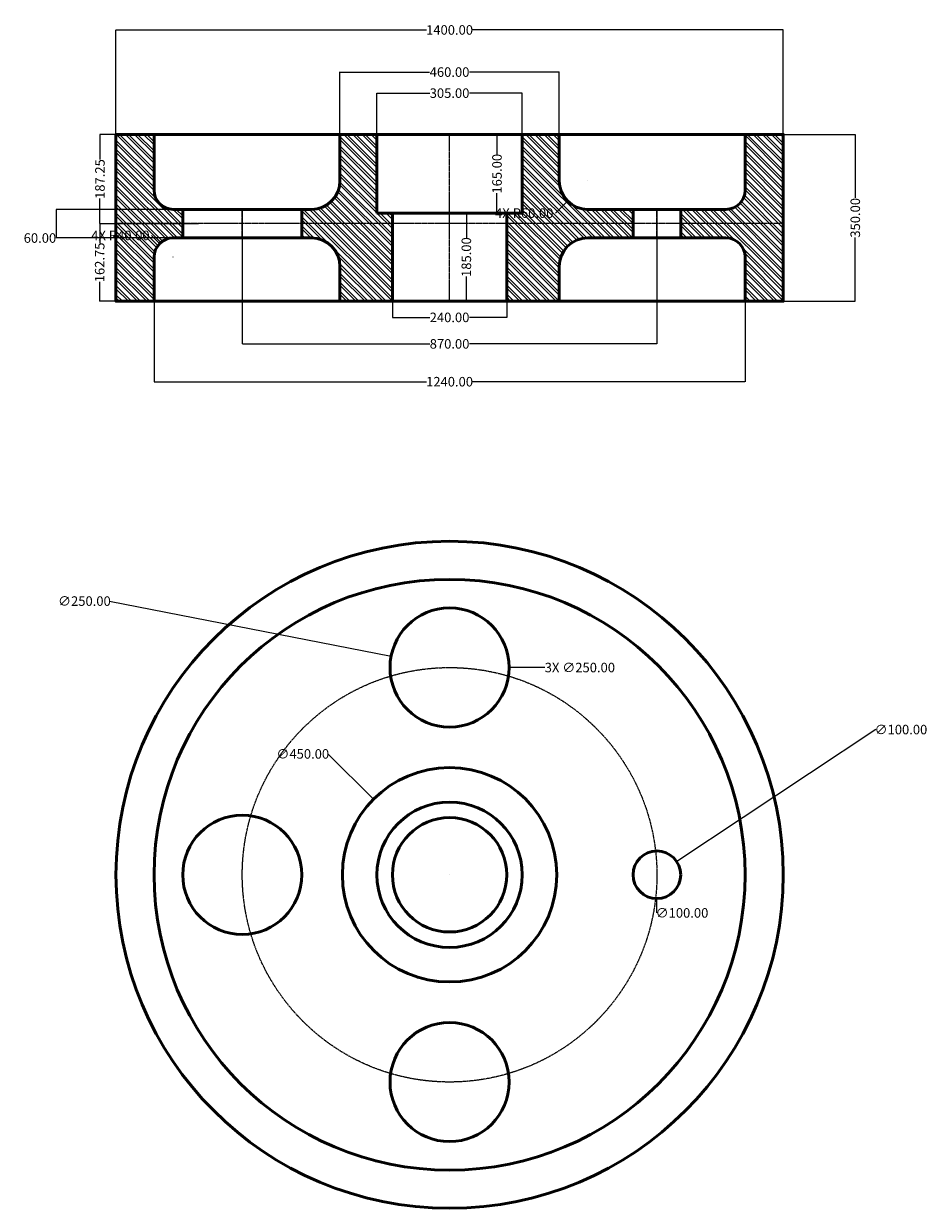
# Model space of a CAD drawing. Units: millimetres. Extents: x -3509 to -1613, y -1694 to 792.
import ezdxf

# ---------------------------------------------------------------- set-up
doc = ezdxf.new("R2010")
doc.units = ezdxf.units.MM
doc.header["$MEASUREMENT"] = 0
doc.linetypes.add('CENTER', pattern=[2, 1.25, -0.25, 0.25, -0.25])
for name, color, linetype, lineweight in [('M-CNTR', 1, 'CENTER', 18), ('M-DIMS', 2, 'Continuous', 25), ('M-HATC', 8, 'Continuous', 18), ('M-OUTL', 7, 'Continuous', 50)]:
    doc.layers.add(name, color=color, linetype=linetype, lineweight=lineweight)
doc.styles.get("Standard").update_dxf_attribs({"font": 'arial.ttf'})
doc.dimstyles.get("Standard").update_dxf_attribs({"dimtxt": 20, "dimasz": 0.18, "dimexe": 0.18, "dimexo": 0.0625, "dimgap": 0.09, "dimtad": 0, "dimtoh": 1, "dimzin": 0, "dimdsep": 46, "dimtxsty": 'Standard', "dimcen": 0.09, "dimadec": 0, "dimazin": 0, "dimtfac": 1, "dimtofl": 0, "dimtmove": 0, "dimatfit": 3, "dimfxl": 1, "dimtolj": 1, "dimtzin": 0, "dimarcsym": 0})

# ---------------------------------------------------------------- blocks, each defined once
blk = doc.blocks.new('*D1')
at = {"layer": 'Defpoints', "color": 0, "transparency": 16777216}
for p in [(-1915.5, 779), (-3315.5, 372.4), (-1915.5, 372.4)]:
    blk.add_point(p, dxfattribs=at)
at = {"layer": 'M-DIMS', "color": 0, "lineweight": -2, "transparency": 16777216}
for p, q in [((-3315.5, 372.5), (-3315.5, 779.2)), ((-3315.3, 779), (-2663.9, 779)), ((-1915.6, 779), (-2567.1, 779)), ((-1915.5, 372.5), (-1915.5, 779.2))]:
    blk.add_line(p, q, dxfattribs=at)
at = {"layer": 'M-DIMS', "color": 0, "transparency": 16777216}
for points in [[(-3315.3, 779), (-3315.3, 779), (-3315.5, 779)], [(-1915.6, 779), (-1915.6, 779), (-1915.5, 779)]]:
    blk.add_solid(points, dxfattribs=at)
at = {"layer": 'M-DIMS', "color": 0, "transparency": 16777216, "insert": (-2615.5, 779), "char_height": 20, "attachment_point": 5}
blk.add_mtext('\\A1;1400.00', dxfattribs=at)
blk = doc.blocks.new('*D2')
at = {"layer": 'Defpoints', "color": 0, "transparency": 16777216}
for p in [(-2385.5, 690.6), (-2845.5, 559.7), (-2385.5, 559.7)]:
    blk.add_point(p, dxfattribs=at)
at = {"layer": 'M-DIMS', "color": 0, "lineweight": -2, "transparency": 16777216}
for p, q in [((-2845.5, 559.7), (-2845.5, 690.8)), ((-2845.3, 690.6), (-2657.4, 690.6)), ((-2385.6, 690.6), (-2573.5, 690.6)), ((-2385.5, 559.7), (-2385.5, 690.8))]:
    blk.add_line(p, q, dxfattribs=at)
at = {"layer": 'M-DIMS', "color": 0, "transparency": 16777216}
for points in [[(-2845.3, 690.6), (-2845.3, 690.6), (-2845.5, 690.6)], [(-2385.6, 690.6), (-2385.6, 690.6), (-2385.5, 690.6)]]:
    blk.add_solid(points, dxfattribs=at)
at = {"layer": 'M-DIMS', "color": 0, "transparency": 16777216, "insert": (-2615.5, 690.6), "char_height": 20, "attachment_point": 5}
blk.add_mtext('\\A1;460.00', dxfattribs=at)
blk = doc.blocks.new('*D3')
at = {"layer": 'Defpoints', "color": 0, "transparency": 16777216}
for p in [(-2463, 646.4), (-2768, 559.7), (-2463, 559.7)]:
    blk.add_point(p, dxfattribs=at)
at = {"layer": 'M-DIMS', "color": 0, "lineweight": -2, "transparency": 16777216}
for p, q in [((-2768, 559.8), (-2768, 646.6)), ((-2463, 559.8), (-2463, 646.6)), ((-2767.8, 646.4), (-2657, 646.4)), ((-2463.1, 646.4), (-2573.9, 646.4))]:
    blk.add_line(p, q, dxfattribs=at)
at = {"layer": 'M-DIMS', "color": 0, "transparency": 16777216}
for points in [[(-2767.8, 646.4), (-2767.8, 646.4), (-2768, 646.4)], [(-2463.1, 646.4), (-2463.1, 646.4), (-2463, 646.4)]]:
    blk.add_solid(points, dxfattribs=at)
at = {"layer": 'M-DIMS', "color": 0, "transparency": 16777216, "insert": (-2615.5, 646.4), "char_height": 20, "attachment_point": 5}
blk.add_mtext('\\A1;305.00', dxfattribs=at)
blk = doc.blocks.new('*D4')
at = {"layer": 'Defpoints', "color": 0, "transparency": 16777216}
for p in [(-2538.9, 559.7), (-2538.9, 394.7), (-2516, 394.7)]:
    blk.add_point(p, dxfattribs=at)
at = {"layer": 'M-DIMS', "color": 0, "lineweight": -2, "transparency": 16777216}
for p, q in [((-2538.8, 559.7), (-2515.8, 559.7)), ((-2516, 559.5), (-2516, 517.8)), ((-2516, 394.9), (-2516, 436.6)), ((-2538.8, 394.7), (-2515.8, 394.7))]:
    blk.add_line(p, q, dxfattribs=at)
at = {"layer": 'M-DIMS', "color": 0, "transparency": 16777216}
for points in [[(-2516, 559.5), (-2516, 559.5), (-2516, 559.7)], [(-2516, 394.9), (-2516, 394.9), (-2516, 394.7)]]:
    blk.add_solid(points, dxfattribs=at)
at = {"layer": 'M-DIMS', "color": 0, "transparency": 16777216, "insert": (-2516, 477.2), "char_height": 20, "attachment_point": 5, "rotation": 90}
blk.add_mtext('\\A1;165.00', dxfattribs=at)
blk = doc.blocks.new('*D5')
at = {"layer": 'Defpoints', "color": 0, "transparency": 16777216}
for p in [(-2538.9, 394.7), (-2580.3, 209.7), (-2538.9, 209.7)]:
    blk.add_point(p, dxfattribs=at)
at = {"layer": 'M-DIMS', "color": 0, "lineweight": -2, "transparency": 16777216}
for p, q in [((-2538.9, 394.7), (-2580.4, 394.7)), ((-2580.3, 394.5), (-2580.3, 342.8)), ((-2580.3, 209.9), (-2580.3, 261.6)), ((-2538.9, 209.7), (-2580.4, 209.7))]:
    blk.add_line(p, q, dxfattribs=at)
at = {"layer": 'M-DIMS', "color": 0, "transparency": 16777216}
for points in [[(-2580.3, 394.5), (-2580.2, 394.5), (-2580.3, 394.7)], [(-2580.3, 209.9), (-2580.2, 209.9), (-2580.3, 209.7)]]:
    blk.add_solid(points, dxfattribs=at)
at = {"layer": 'M-DIMS', "color": 0, "transparency": 16777216, "insert": (-2580.3, 302.2), "char_height": 20, "attachment_point": 5, "rotation": 90}
blk.add_mtext('\\A1;185.00', dxfattribs=at)
blk = doc.blocks.new('*D6')
at = {"layer": 'Defpoints', "color": 0, "transparency": 16777216}
for p in [(-2735.5, 209.7), (-2495.5, 209.7), (-2495.5, 175.7)]:
    blk.add_point(p, dxfattribs=at)
at = {"layer": 'M-DIMS', "color": 0, "lineweight": -2, "transparency": 16777216}
for p, q in [((-2735.5, 209.6), (-2735.5, 175.5)), ((-2495.5, 209.6), (-2495.5, 175.5)), ((-2735.3, 175.7), (-2657.2, 175.7)), ((-2495.6, 175.7), (-2573.7, 175.7))]:
    blk.add_line(p, q, dxfattribs=at)
at = {"layer": 'M-DIMS', "color": 0, "transparency": 16777216}
for points in [[(-2735.3, 175.7), (-2735.3, 175.6), (-2735.5, 175.7)], [(-2495.6, 175.7), (-2495.6, 175.6), (-2495.5, 175.7)]]:
    blk.add_solid(points, dxfattribs=at)
at = {"layer": 'M-DIMS', "color": 0, "transparency": 16777216, "insert": (-2615.5, 175.7), "char_height": 20, "attachment_point": 5}
blk.add_mtext('\\A1;240.00', dxfattribs=at)
blk = doc.blocks.new('*D7')
at = {"layer": 'Defpoints', "color": 0, "transparency": 16777216}
for p in [(-3050.5, 402.4), (-2180.5, 402.4), (-2180.5, 120.1)]:
    blk.add_point(p, dxfattribs=at)
at = {"layer": 'M-DIMS', "color": 0, "lineweight": -2, "transparency": 16777216}
for p, q in [((-3050.5, 402.4), (-3050.5, 119.9)), ((-2180.5, 402.4), (-2180.5, 119.9)), ((-3050.3, 120.1), (-2657, 120.1)), ((-2180.6, 120.1), (-2573.9, 120.1))]:
    blk.add_line(p, q, dxfattribs=at)
at = {"layer": 'M-DIMS', "color": 0, "transparency": 16777216}
for points in [[(-3050.3, 120.1), (-3050.3, 120), (-3050.5, 120.1)], [(-2180.6, 120.1), (-2180.6, 120), (-2180.5, 120.1)]]:
    blk.add_solid(points, dxfattribs=at)
at = {"layer": 'M-DIMS', "color": 0, "transparency": 16777216, "insert": (-2615.5, 120.1), "char_height": 20, "attachment_point": 5}
blk.add_mtext('\\A1;870.00', dxfattribs=at)
blk = doc.blocks.new('*D8')
at = {"layer": 'Defpoints', "color": 0, "transparency": 16777216}
for p in [(-3235.5, 209.7), (-1995.5, 209.7), (-1995.5, 40.7)]:
    blk.add_point(p, dxfattribs=at)
at = {"layer": 'M-DIMS', "color": 0, "lineweight": -2, "transparency": 16777216}
for p, q in [((-3235.5, 209.6), (-3235.5, 40.5)), ((-1995.5, 209.6), (-1995.5, 40.5)), ((-3235.3, 40.7), (-2663.9, 40.7)), ((-1995.6, 40.7), (-2567.1, 40.7))]:
    blk.add_line(p, q, dxfattribs=at)
at = {"layer": 'M-DIMS', "color": 0, "transparency": 16777216}
for points in [[(-3235.3, 40.7), (-3235.3, 40.6), (-3235.5, 40.7)], [(-1995.6, 40.7), (-1995.6, 40.6), (-1995.5, 40.7)]]:
    blk.add_solid(points, dxfattribs=at)
at = {"layer": 'M-DIMS', "color": 0, "transparency": 16777216, "insert": (-2615.5, 40.7), "char_height": 20, "attachment_point": 5}
blk.add_mtext('\\A1;1240.00', dxfattribs=at)
blk = doc.blocks.new('*D9')
at = {"layer": 'Defpoints', "color": 0, "transparency": 16777216}
for p in [(-1915.5, 559.7), (-1915.5, 209.7), (-1764.2, 209.7)]:
    blk.add_point(p, dxfattribs=at)
at = {"layer": 'M-DIMS', "color": 0, "lineweight": -2, "transparency": 16777216}
for p, q in [((-1915.4, 559.7), (-1764.1, 559.7)), ((-1764.2, 559.5), (-1764.2, 426.3)), ((-1764.2, 209.9), (-1764.2, 343.1)), ((-1915.4, 209.7), (-1764.1, 209.7))]:
    blk.add_line(p, q, dxfattribs=at)
at = {"layer": 'M-DIMS', "color": 0, "transparency": 16777216}
for points in [[(-1764.3, 559.5), (-1764.2, 559.5), (-1764.2, 559.7)], [(-1764.3, 209.9), (-1764.2, 209.9), (-1764.2, 209.7)]]:
    blk.add_solid(points, dxfattribs=at)
at = {"layer": 'M-DIMS', "color": 0, "transparency": 16777216, "insert": (-1764.2, 384.7), "char_height": 20, "attachment_point": 5, "rotation": 90}
blk.add_mtext('\\A1;350.00', dxfattribs=at)
blk = doc.blocks.new('*D10')
at = {"layer": 'Defpoints', "color": 0, "transparency": 16777216}
for p in [(-2738.1, -535.2), (-2492.8, -583.2)]:
    blk.add_point(p, dxfattribs=at)
at = {"layer": 'M-DIMS', "color": 0, "lineweight": -2, "transparency": 16777216}
for p, q in [((-3329.2, -419.7), (-2738.3, -535.2)), ((-2615.5, -559.3), (-2615.5, -559.1)), ((-2615.5, -559.2), (-2615.4, -559.2))]:
    blk.add_line(p, q, dxfattribs=at)
at = {"layer": 'M-DIMS', "color": 0, "transparency": 16777216}
blk.add_solid([(-2738.3, -535.2), (-2738.3, -535.2), (-2738.1, -535.2)], dxfattribs=at)
at = {"layer": 'M-DIMS', "color": 0, "transparency": 16777216, "insert": (-3381.7, -419.7), "char_height": 20, "attachment_point": 5}
blk.add_mtext('\\A1;∅250.00', dxfattribs=at)
blk = doc.blocks.new('*D11')
at = {"layer": 'Defpoints', "color": 0, "transparency": 16777216}
for p in [(-2138.8, -966.6), (-2222.1, -1021.8)]:
    blk.add_point(p, dxfattribs=at)
at = {"layer": 'M-DIMS', "color": 0, "lineweight": -2, "transparency": 16777216}
for p, q in [((-1721, -689.4), (-2138.6, -966.5)), ((-1720.8, -689.4), (-1721, -689.4)), ((-2180.5, -994.3), (-2180.5, -994.1)), ((-2180.5, -994.2), (-2180.4, -994.2))]:
    blk.add_line(p, q, dxfattribs=at)
at = {"layer": 'M-DIMS', "color": 0, "transparency": 16777216}
blk.add_solid([(-2138.7, -966.4), (-2138.6, -966.5), (-2138.8, -966.6)], dxfattribs=at)
at = {"layer": 'M-DIMS', "color": 0, "transparency": 16777216, "insert": (-1668.4, -689.4), "char_height": 20, "attachment_point": 5}
blk.add_mtext('\\A1;∅100.00', dxfattribs=at)
blk = doc.blocks.new('*D12')
at = {"layer": 'Defpoints', "color": 0, "transparency": 16777216}
for p in [(-3278, 559.7), (-3349.1, 372.4), (-3278, 372.4)]:
    blk.add_point(p, dxfattribs=at)
at = {"layer": 'M-DIMS', "color": 0, "lineweight": -2, "transparency": 16777216}
for p, q in [((-3278.1, 559.7), (-3349.2, 559.7)), ((-3349.1, 559.5), (-3349.1, 506.8)), ((-3349.1, 372.6), (-3349.1, 425.3)), ((-3278.1, 372.4), (-3349.2, 372.4))]:
    blk.add_line(p, q, dxfattribs=at)
at = {"layer": 'M-DIMS', "color": 0, "transparency": 16777216}
for points in [[(-3349.1, 559.5), (-3349, 559.5), (-3349.1, 559.7)], [(-3349.1, 372.6), (-3349, 372.6), (-3349.1, 372.4)]]:
    blk.add_solid(points, dxfattribs=at)
at = {"layer": 'M-DIMS', "color": 0, "transparency": 16777216, "insert": (-3349.1, 466.1), "char_height": 20, "attachment_point": 5, "rotation": 90}
blk.add_mtext('\\A1;187.25', dxfattribs=at)
blk = doc.blocks.new('*D13')
at = {"layer": 'Defpoints', "color": 0, "transparency": 16777216}
for p in [(-3142.5, 372.4), (-3349.6, 209.7), (-3142.5, 209.7)]:
    blk.add_point(p, dxfattribs=at)
at = {"layer": 'M-DIMS', "color": 0, "lineweight": -2, "transparency": 16777216}
for p, q in [((-3142.6, 372.4), (-3349.8, 372.4)), ((-3349.6, 372.3), (-3349.6, 331.8)), ((-3349.6, 209.9), (-3349.6, 250.3)), ((-3142.6, 209.7), (-3349.8, 209.7))]:
    blk.add_line(p, q, dxfattribs=at)
at = {"layer": 'M-DIMS', "color": 0, "transparency": 16777216}
for points in [[(-3349.6, 372.3), (-3349.5, 372.3), (-3349.6, 372.4)], [(-3349.6, 209.9), (-3349.5, 209.9), (-3349.6, 209.7)]]:
    blk.add_solid(points, dxfattribs=at)
at = {"layer": 'M-DIMS', "color": 0, "transparency": 16777216, "insert": (-3349.6, 291.1), "char_height": 20, "attachment_point": 5, "rotation": 90}
blk.add_mtext('\\A1;162.75', dxfattribs=at)
blk = doc.blocks.new('*D14')
at = {"layer": 'Defpoints', "color": 0, "transparency": 16777216}
for p in [(-2925.5, 402.4), (-3441, 342.4), (-2925.5, 342.4)]:
    blk.add_point(p, dxfattribs=at)
at = {"layer": 'M-DIMS', "color": 0, "lineweight": -2, "transparency": 16777216}
for p, q in [((-2925.5, 402.4), (-3441.1, 402.4)), ((-3441, 402.3), (-3441, 342.6)), ((-2925.5, 342.4), (-3441.1, 342.4)), ((-3441, 342.3), (-3441.1, 342.3)), ((-3441, 342.4), (-3441, 342.3))]:
    blk.add_line(p, q, dxfattribs=at)
at = {"layer": 'M-DIMS', "color": 0, "transparency": 16777216}
for points in [[(-3441, 402.3), (-3440.9, 402.3), (-3441, 402.4)], [(-3441, 342.6), (-3440.9, 342.6), (-3441, 342.4)]]:
    blk.add_solid(points, dxfattribs=at)
at = {"layer": 'M-DIMS', "color": 0, "transparency": 16777216, "insert": (-3475, 342.3), "char_height": 20, "attachment_point": 5}
blk.add_mtext('\\A1;60.00', dxfattribs=at)
blk = doc.blocks.new('*D15')
at = {"layer": 'Defpoints', "color": 0, "transparency": 16777216}
for p in [(-3223.7, 330.7), (-3195.5, 302.4)]:
    blk.add_point(p, dxfattribs=at)
at = {"layer": 'M-DIMS', "color": 0, "lineweight": -2, "transparency": 16777216}
for p, q in [((-3240.9, 347.7), (-3240.7, 347.7)), ((-3240.7, 347.7), (-3223.9, 330.9)), ((-3195.5, 302.4), (-3195.5, 302.5)), ((-3195.5, 302.4), (-3195.4, 302.4))]:
    blk.add_line(p, q, dxfattribs=at)
at = {"layer": 'M-DIMS', "color": 0, "transparency": 16777216}
blk.add_solid([(-3223.8, 330.9), (-3223.9, 330.8), (-3223.7, 330.7)], dxfattribs=at)
at = {"layer": 'M-DIMS', "color": 0, "transparency": 16777216, "insert": (-3306.1, 347.7), "char_height": 20, "attachment_point": 5}
blk.add_mtext('\\A1;4X R40.00', dxfattribs=at)
blk = doc.blocks.new('*D16')
at = {"layer": 'Defpoints', "color": 0, "transparency": 16777216}
for p in [(-2325.5, 462.4), (-2367.9, 420)]:
    blk.add_point(p, dxfattribs=at)
at = {"layer": 'M-DIMS', "color": 0, "lineweight": -2, "transparency": 16777216}
for p, q in [((-2325.5, 462.4), (-2325.5, 462.5)), ((-2325.5, 462.4), (-2325.4, 462.4)), ((-2393.3, 394.6), (-2368, 419.9)), ((-2393.5, 394.6), (-2393.3, 394.6))]:
    blk.add_line(p, q, dxfattribs=at)
at = {"layer": 'M-DIMS', "color": 0, "transparency": 16777216}
blk.add_solid([(-2368, 419.9), (-2368, 419.9), (-2367.9, 420)], dxfattribs=at)
at = {"layer": 'M-DIMS', "color": 0, "transparency": 16777216, "insert": (-2458.8, 394.6), "char_height": 20, "attachment_point": 5}
blk.add_mtext('\\A1;4X R60.00', dxfattribs=at)
blk = doc.blocks.new('*D17')
at = {"layer": 'Defpoints', "color": 0, "transparency": 16777216}
for p in [(-2740.5, -559.2), (-2490.5, -559.2)]:
    blk.add_point(p, dxfattribs=at)
at = {"layer": 'M-DIMS', "color": 0, "lineweight": -2, "transparency": 16777216}
for p, q in [((-2615.5, -559.3), (-2615.5, -559.1)), ((-2615.5, -559.2), (-2615.4, -559.2)), ((-2415.5, -559.2), (-2490.3, -559.2))]:
    blk.add_line(p, q, dxfattribs=at)
at = {"layer": 'M-DIMS', "color": 0, "transparency": 16777216}
blk.add_solid([(-2490.3, -559.2), (-2490.3, -559.2), (-2490.5, -559.2)], dxfattribs=at)
at = {"layer": 'M-DIMS', "color": 0, "transparency": 16777216, "insert": (-2342.1, -559.2), "char_height": 20, "attachment_point": 5}
blk.add_mtext('\\A1;3X ∅250.00', dxfattribs=at)
blk = doc.blocks.new('*D18')
at = {"layer": 'Defpoints', "color": 0, "transparency": 16777216}
for p in [(-2180.5, -944.2), (-2180.5, -1044.2)]:
    blk.add_point(p, dxfattribs=at)
at = {"layer": 'M-DIMS', "color": 0, "lineweight": -2, "transparency": 16777216}
for p, q in [((-2180.5, -994.3), (-2180.5, -994.1)), ((-2180.5, -994.2), (-2180.4, -994.2)), ((-2180.5, -1074.2), (-2180.5, -1044.4)), ((-2180.3, -1074.2), (-2180.5, -1074.2))]:
    blk.add_line(p, q, dxfattribs=at)
at = {"layer": 'M-DIMS', "color": 0, "transparency": 16777216}
blk.add_solid([(-2180.4, -1044.4), (-2180.5, -1044.4), (-2180.5, -1044.2)], dxfattribs=at)
at = {"layer": 'M-DIMS', "color": 0, "transparency": 16777216, "insert": (-2127.8, -1074.2), "char_height": 20, "attachment_point": 5}
blk.add_mtext('\\A1;∅100.00', dxfattribs=at)
blk = doc.blocks.new('*D19')
at = {"layer": 'Defpoints', "color": 0, "transparency": 16777216}
for p in [(-2775.1, -835.6), (-2455.8, -1152.8)]:
    blk.add_point(p, dxfattribs=at)
at = {"layer": 'M-DIMS', "color": 0, "lineweight": -2, "transparency": 16777216}
for p, q in [((-2871, -740.5), (-2870.8, -740.5)), ((-2870.8, -740.5), (-2775.2, -835.5)), ((-2615.5, -994.3), (-2615.5, -994.1)), ((-2615.5, -994.2), (-2615.4, -994.2))]:
    blk.add_line(p, q, dxfattribs=at)
at = {"layer": 'M-DIMS', "color": 0, "transparency": 16777216}
blk.add_solid([(-2775.2, -835.5), (-2775.2, -835.5), (-2775.1, -835.6)], dxfattribs=at)
at = {"layer": 'M-DIMS', "color": 0, "transparency": 16777216, "insert": (-2923.5, -740.5), "char_height": 20, "attachment_point": 5}
blk.add_mtext('\\A1;∅450.00', dxfattribs=at)

msp = doc.modelspace()

# ---------------------------------------------------------------- hatches: boundary and pattern name
at = {"layer": 'M-HATC'}
h = msp.add_hatch(dxfattribs=at)
h.set_pattern_fill('ANSI32', color=256, scale=36, angle=90)
h.set_pattern_definition([(135, (-3499.538, 0), (-9.54594, -9.54594), []), (135, (-3499.538, 6.364), (-9.54594, -9.54594), [])])
h.paths.add_polyline_path([(-3235.455, 559.695), (-3315.455, 559.695), (-3315.455, 372.445), (-3175.455, 372.445), (-3175.455, 402.445), (-3195.455, 402.445, -0.41421356), (-3235.455, 442.445)])
h.paths.add_polyline_path([(-3195.455, 342.445), (-3175.455, 342.445), (-3175.455, 372.445), (-3315.455, 372.445), (-3315.455, 209.695), (-3235.455, 209.695), (-3235.455, 302.445, -0.41421356)])
h.paths.add_polyline_path([(-2767.955, 559.695), (-2845.455, 559.695), (-2845.455, 462.445, -0.41421356), (-2905.455, 402.445), (-2925.455, 402.445), (-2925.455, 372.445), (-2735.455, 372.445), (-2735.455, 394.695), (-2767.955, 394.695)])
h.paths.add_polyline_path([(-2735.455, 372.445), (-2925.455, 372.445), (-2925.455, 342.445), (-2905.455, 342.445, -0.41421356), (-2845.455, 282.445), (-2845.455, 209.695), (-2735.455, 209.695)])
h.paths.add_polyline_path([(-2325.455, 342.445), (-2230.455, 342.445), (-2230.455, 372.445), (-2495.455, 372.445), (-2495.455, 209.695), (-2385.455, 209.695), (-2385.455, 282.445, -0.41421356)])
h.paths.add_polyline_path([(-2385.455, 462.445), (-2385.455, 559.695), (-2462.955, 559.695), (-2462.955, 394.695), (-2495.455, 394.695), (-2495.455, 372.445), (-2230.455, 372.445), (-2230.455, 402.445), (-2325.455, 402.445, -0.41421356)])
h.paths.add_polyline_path([(-1915.455, 559.695), (-1995.455, 559.695), (-1995.455, 442.445, -0.41421356), (-2035.455, 402.445), (-2130.455, 402.445), (-2130.455, 372.445), (-1915.455, 372.445)])
h.paths.add_polyline_path([(-1915.455, 372.445), (-2130.455, 372.445), (-2130.455, 342.445), (-2035.455, 342.445, -0.41421356), (-1995.455, 302.445), (-1995.455, 209.695), (-1915.455, 209.695)])

# ---------------------------------------------------------------- linework, layer by layer
at = {"layer": 'M-CNTR'}
for p, q in [((-2615.455, 559.695), (-2615.455, 559.815)), ((-2615.455, 209.575), (-2615.455, 559.815)), ((-3050.455, 342.445), (-3050.455, 402.445)), ((-2180.455, 342.445), (-2180.455, 402.445)), ((-1915.455, 372.445), (-3315.455, 372.445)), ((-2615.455, 209.575), (-2615.455, 209.695))]:
    msp.add_line(p, q, dxfattribs=at)
msp.add_circle((-2615.455, -994.199), 435, dxfattribs=at)
at = {"layer": 'M-OUTL'}
for p, q in [((-3235.455, 559.695), (-3235.455, 442.445)), ((-2845.455, 559.683), (-2845.455, 462.445)), ((-2767.955, 559.695), (-2767.955, 394.695)), ((-2462.955, 394.695), (-2462.955, 559.695)), ((-2385.455, 559.695), (-2385.455, 462.445)), ((-1995.455, 559.62), (-1995.455, 442.445)), ((-2905.455, 402.445), (-3195.455, 402.445)), ((-3175.455, 342.445), (-3175.455, 402.445)), ((-2925.455, 342.445), (-2925.455, 402.445)), ((-2035.455, 402.445), (-2325.455, 402.445)), ((-2230.455, 342.445), (-2230.455, 402.445)), ((-2130.455, 342.445), (-2130.455, 402.445)), ((-2767.955, 394.695), (-2462.955, 394.695)), ((-2735.455, 209.695), (-2735.455, 394.695)), ((-2735.455, 394.695), (-2495.455, 394.695)), ((-2495.455, 394.695), (-2495.455, 209.695)), ((-2905.455, 342.445), (-3195.455, 342.445)), ((-2035.455, 342.445), (-2325.455, 342.445)), ((-3235.455, 302.445), (-3235.455, 209.695)), ((-1995.455, 302.445), (-1995.455, 209.695)), ((-2845.455, 282.445), (-2845.455, 209.695)), ((-2385.455, 282.445), (-2385.455, 209.695))]:
    msp.add_line(p, q, dxfattribs=at)
msp.add_lwpolyline([(-3315.455, 559.695), (-1915.455, 559.695), (-1915.455, 209.695), (-3315.455, 209.695)], close=True, dxfattribs=at)
for centre, radius in [((-2615.455, -994.199), 700), ((-2615.455, -994.199), 620), ((-2615.455, -559.199), 125), ((-2615.455, -994.199), 225), ((-2615.455, -994.199), 152.5), ((-3050.455, -994.199), 125), ((-2615.455, -994.199), 120), ((-2180.455, -994.199), 50), ((-2615.455, -1429.199), 125)]:
    msp.add_circle(centre, radius, dxfattribs=at)
for centre, radius, start, end in [((-2905.455, 462.445), 60, 270, 0), ((-2325.455, 462.445), 60, 180, 270), ((-3195.455, 442.445), 40, 180, 270), ((-2035.455, 442.445), 40, 270, 0), ((-3195.455, 302.445), 40, 90, 180), ((-2905.455, 282.445), 60, 0, 90), ((-2325.455, 282.445), 60, 90, 180), ((-2035.455, 302.445), 40, 0, 90)]:
    msp.add_arc(centre, radius, start, end, dxfattribs=at)

# ---------------------------------------------------------------- dimensions: what is measured, and where the dimension line sits
at = {"layer": 'M-DIMS'}
for base, p1, p2, picture, middle in [((-1915.455, 779), (-3315.455, 372.445), (-1915.455, 372.445), '*D1', (-2615.455, 779)), ((-2385.455, 690.603), (-2845.455, 559.683), (-2385.455, 559.683), '*D2', (-2615.455, 690.603)), ((-2462.955, 646.405), (-2767.955, 559.695), (-2462.955, 559.695), '*D3', (-2615.455, 646.405)), ((-2180.455, 120.073), (-3050.455, 402.445), (-2180.455, 402.445), '*D7', (-2615.455, 120.073)), ((-1995.455, 40.658), (-3235.455, 209.695), (-1995.455, 209.695), '*D8', (-2615.455, 40.658)), ((-2495.455, 175.677), (-2735.455, 209.695), (-2495.455, 209.695), '*D6', (-2615.455, 175.677))]:
    dim = msp.add_linear_dim(base=base, p1=p1, p2=p2, dimstyle='Standard', override={"dimclrd": 0, "dimclre": 0, "dimclrt": 0}, dxfattribs=at)
    dim.commit()
    dim.dimension.update_dxf_attribs({"geometry": picture, "text_midpoint": middle})
for base, p1, p2, override, picture, middle in [((-3349.057, 372.445), (-3278.011, 559.695), (-3278.011, 372.445), {"dimclrd": 0, "dimclre": 0, "dimclrt": 0}, '*D12', (-3349.057, 466.07)), ((-2516.017, 394.695), (-2538.86, 559.695), (-2538.86, 394.695), {"dimclrd": 0, "dimclre": 0, "dimclrt": 0}, '*D4', (-2516.017, 477.195)), ((-1764.235, 209.695), (-1915.455, 559.695), (-1915.455, 209.695), {"dimclrd": 0, "dimclre": 0, "dimclrt": 0}, '*D9', (-1764.235, 384.695)), ((-3440.955, 342.445), (-2925.455, 402.445), (-2925.455, 342.445), {"dimdec": 2, "dimlfac": 1, "dimrnd": 0, "dimzin": 0, "dimdsep": 46, "dimlunit": 2}, '*D14', (-3474.991, 342.265)), ((-2580.26, 209.695), (-2538.86, 394.695), (-2538.86, 209.695), {"dimclrd": 0, "dimclre": 0, "dimclrt": 0}, '*D5', (-2580.26, 302.195)), ((-3349.575, 209.695), (-3142.546, 372.445), (-3142.546, 209.695), {"dimclrd": 0, "dimclre": 0, "dimclrt": 0}, '*D13', (-3349.575, 291.07))]:
    dim = msp.add_linear_dim(base=base, p1=p1, p2=p2, angle=90, dimstyle='Standard', override=override, dxfattribs=at)
    dim.commit()
    dim.dimension.update_dxf_attribs({"geometry": picture, "text_midpoint": middle})
for center, mpoint, picture, middle in [((-2325.455, 462.445), (-2367.882, 420.019), '*D16', (-2458.778, 394.563)), ((-3195.455, 302.445), (-3223.739, 330.73), '*D15', (-3306.15, 347.701))]:
    dim = msp.add_radius_dim(center=center, mpoint=mpoint, text='4X <>', dimstyle='Standard', override={"dimdec": 2, "dimlfac": 1, "dimrnd": 0, "dimzin": 0, "dimdsep": 46, "dimlunit": 2}, dxfattribs=at)
    dim.commit()
    dim.dimension.update_dxf_attribs({"geometry": picture, "text_midpoint": middle, "dimtype": 164})
for p1, p2, override, picture, middle in [((-2492.775, -583.169), (-2738.135, -535.229), {"dimclrd": 0, "dimclre": 0, "dimclrt": 0}, '*D10', (-3329.24, -419.735)), ((-2222.121, -1021.839), (-2138.79, -966.559), {"dimclrd": 0, "dimclre": 0, "dimclrt": 0}, '*D11', (-1668.36, -689.401)), ((-2455.836, -1152.775), (-2775.075, -835.622), {"dimdec": 2, "dimlfac": 1, "dimrnd": 0, "dimzin": 0, "dimdsep": 46, "dimlunit": 2}, '*D19', (-2923.477, -740.476)), ((-2180.455, -944.199), (-2180.455, -1044.199), {"dimdec": 2, "dimlfac": 1, "dimrnd": 0, "dimzin": 0, "dimdsep": 46, "dimlunit": 2}, '*D18', (-2127.825, -1074.199))]:
    dim = msp.add_diameter_dim_2p(p1=p1, p2=p2, dimstyle='Standard', override=override, dxfattribs=at)
    dim.commit()
    dim.dimension.update_dxf_attribs({"geometry": picture, "text_midpoint": middle, "dimtype": 163})
dim = msp.add_diameter_dim_2p(p1=(-2740.455, -559.198), p2=(-2490.455, -559.199), text='3X <>', dimstyle='Standard', override={"dimdec": 2, "dimlfac": 1, "dimrnd": 0, "dimzin": 0, "dimdsep": 46, "dimlunit": 2}, dxfattribs=at)
dim.commit()
dim.dimension.update_dxf_attribs({"geometry": '*D17', "text_midpoint": (-2415.455, -559.199), "dimtype": 163})

doc.saveas('drawing.dxf')
